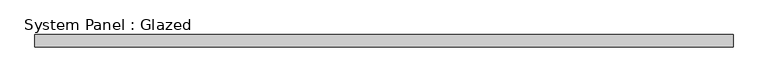
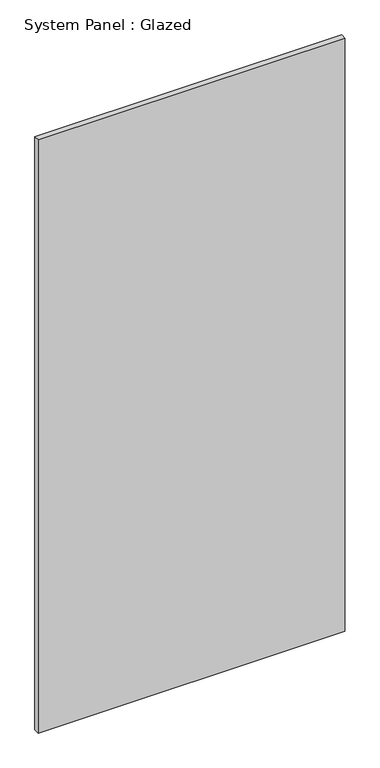
"""IFC4 building model written with IfcOpenShell, lengths in millimetres: plate geometry, System Panel : Glazed."""

from ifc_helpers import new_model, si_unit, origin, origin_with_axes, place, context, project, spatial, polyline, outline, extrude, source, transform, mapped, element, save


def system_panel_glazed_70f543ca(model_context):
    return source(origin(), model_context, "Body", "SweptSolid", [
        extrude(outline(polyline([(714.375, 19.05), (-714.375, 19.05), (-714.375, 44.45), (714.375, 44.45), (714.375, 19.05)])), origin_with_axes(), (0.0, 0.0, 1.0), 2921.0),
    ])


if __name__ == "__main__":
    model = new_model("IFC4")
    model_context = context("Model", 3, world=origin())
    ifc_project = project(units=[si_unit("LENGTHUNIT", "METRE", prefix="MILLI")], contexts=[model_context])
    site = spatial("IfcSite", under=ifc_project)
    building = spatial("IfcBuilding", under=site)
    placement = place(None, origin())
    system_panel_glazed_shape = system_panel_glazed_70f543ca(model_context)
    element("IfcPlate", 1, ObjectType="System Panel : Glazed", at=placement, inside=building, context=model_context, shape_type="MappedRepresentation", body=[
        mapped(system_panel_glazed_shape, transform((0.0, 0.0, 0.0), x_axis=(1.0, 0.0, 0.0), y_axis=(0.0, 1.0, 0.0), z_axis=(0.0, 0.0, 1.0))),
    ])
    save(model, "model.ifc")

# Revit data of these elements
# Type "System Panel : Glazed"
#   Construction Type Id = "GSP4R"
#   Analytic Construction = "1/8 in Pilkington single glazing"
#   Visual Light Transmittance = 0.9
#   Solar Heat Gain Coefficient = 0.86
#   Heat Transfer Coefficient (U) = 1.18115 BTU/(h·ft²·°F)
# Element 1 (IfcPlate, "System Panel : Glazed")
#   Materials on its faces: "Glass"
# Materials
#   "Glass": class "Glass", colour RGB 0 128 192, transparency 0.75, Description = "Soda Lime Glass", Cost = 0
